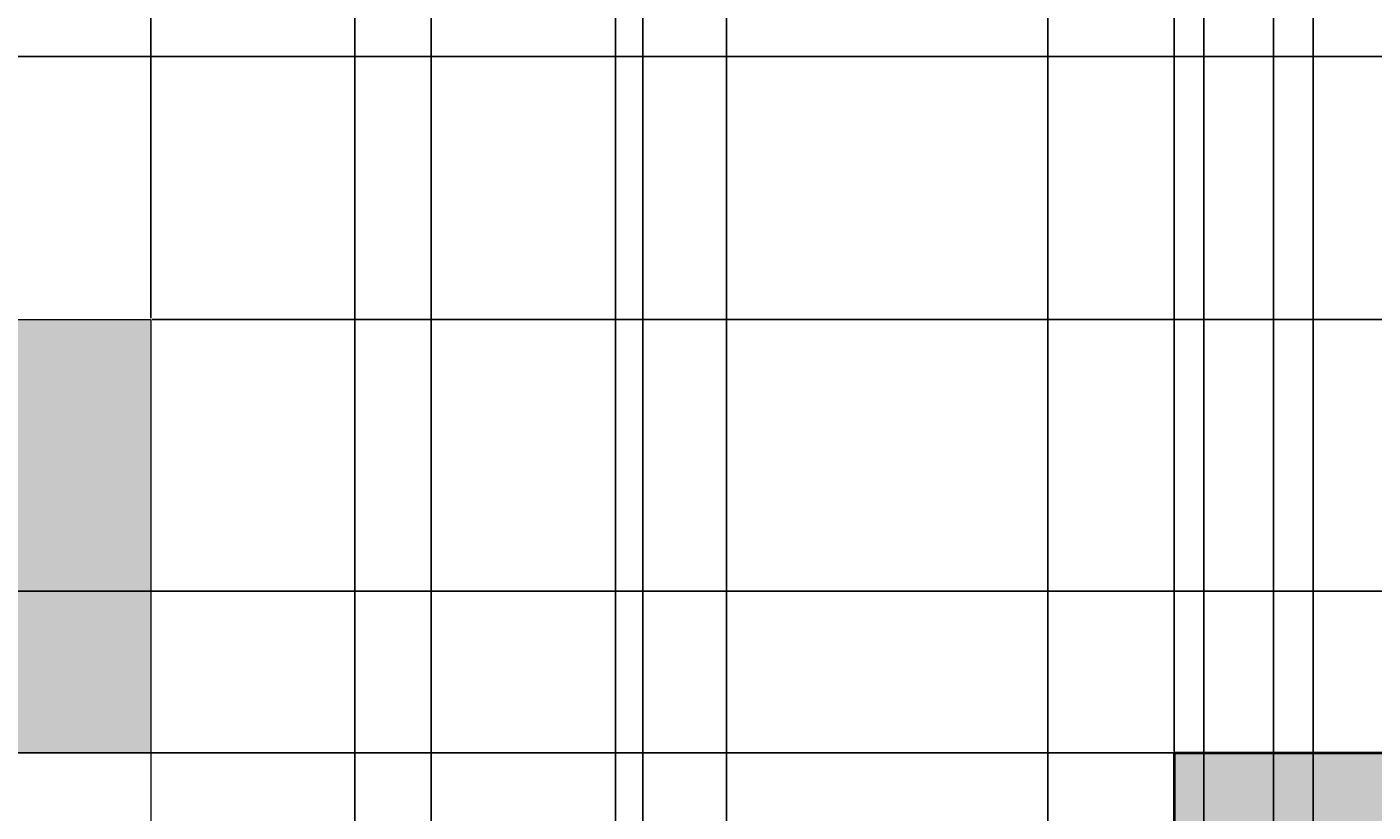
# Model space of a CAD drawing. Units: inches. Extents: x 818 to 1898, y 976 to 2364.
# Tile 70 of 96: x 1372 to 1439, y 1873 to 1913. Entities that reach past the tile are written whole.
import ezdxf

# ---------------------------------------------------------------- set-up
doc = ezdxf.new("R2010")
doc.units = ezdxf.units.IN
doc.header["$LTSCALE"] = 5
doc.header["$MEASUREMENT"] = 0
for name, color, linetype, lineweight in [('A-ANNO-DIMS', 2, 'Continuous', 18), ('A-FLOR-CASE', 8, 'Continuous', 18), ('A-FURN-PATT', 8, 'Continuous', 9), ('A-WALL', 7, 'Continuous', 40)]:
    doc.layers.add(name, color=color, linetype=linetype, lineweight=lineweight)
doc.layers.add('A-WALL-PATT', color=251, linetype='Continuous', lineweight=13, true_color=0x636466)
doc.styles.get("Standard").update_dxf_attribs({"font": 'arial.ttf'})
doc.dimstyles.get("Standard").update_dxf_attribs({"dimtxt": 0.18, "dimasz": 0.18, "dimexe": 0.18, "dimexo": 0.0625, "dimgap": 0.09, "dimtad": 0, "dimtih": 1, "dimtoh": 1, "dimdec": 4, "dimzin": 0, "dimdsep": 46, "dimtxsty": 'Standard', "dimcen": 0.09, "dimadec": 0, "dimazin": 0, "dimtfac": 1, "dimtdec": 4, "dimtofl": 0, "dimtmove": 0, "dimatfit": 3, "dimfxl": 1, "dimtolj": 1, "dimtzin": 0, "dimarcsym": 0})

# ---------------------------------------------------------------- blocks, each defined once
blk = doc.blocks.new('*D61')
at = {"layer": 'A-ANNO-DIMS', "color": 0, "lineweight": -2, "ltscale": 5, "transparency": 16777216}
for p, q in [((1071.725, 1203.027), (1071.725, 2363.873)), ((1071.905, 2363.693), (1250.936, 2363.693)), ((1430.545, 2363.693), (1251.514, 2363.693)), ((1430.725, 1203.027), (1430.725, 2363.873))]:
    blk.add_line(p, q, dxfattribs=at)
at = {"layer": 'A-ANNO-DIMS', "color": 0, "ltscale": 5, "transparency": 16777216}
for points in [[(1071.905, 2363.723), (1071.905, 2363.663), (1071.725, 2363.693)], [(1430.545, 2363.723), (1430.545, 2363.663), (1430.725, 2363.693)]]:
    blk.add_solid(points, dxfattribs=at)
at = {"layer": 'Defpoints', "color": 0, "ltscale": 5, "transparency": 16777216}
for p in [(1430.725, 2363.693), (1071.725, 1202.964), (1430.725, 1202.964)]:
    blk.add_point(p, dxfattribs=at)
at = {"layer": 'A-ANNO-DIMS', "color": 0, "ltscale": 5, "transparency": 16777216, "insert": (1251.225, 2363.693), "char_height": 0.18, "attachment_point": 5}
blk.add_mtext('\\A1;359', dxfattribs=at)
blk = doc.blocks.new('*D64')
at = {"layer": 'A-ANNO-DIMS', "color": 0, "lineweight": -2, "ltscale": 5, "transparency": 16777216}
for p, q in [((1197.725, 1501.141), (1197.725, 2363.873)), ((1197.905, 2363.693), (1313.935, 2363.693)), ((1430.545, 2363.693), (1314.516, 2363.693)), ((1430.725, 1501.141), (1430.725, 2363.873))]:
    blk.add_line(p, q, dxfattribs=at)
at = {"layer": 'A-ANNO-DIMS', "color": 0, "ltscale": 5, "transparency": 16777216}
for points in [[(1197.905, 2363.723), (1197.905, 2363.663), (1197.725, 2363.693)], [(1430.545, 2363.723), (1430.545, 2363.663), (1430.725, 2363.693)]]:
    blk.add_solid(points, dxfattribs=at)
at = {"layer": 'Defpoints', "color": 0, "ltscale": 5, "transparency": 16777216}
for p in [(1430.725, 2363.693), (1197.725, 1501.078), (1430.725, 1501.078)]:
    blk.add_point(p, dxfattribs=at)
at = {"layer": 'A-ANNO-DIMS', "color": 0, "ltscale": 5, "transparency": 16777216, "insert": (1314.225, 2363.693), "char_height": 0.18, "attachment_point": 5}
blk.add_mtext('\\A1;233', dxfattribs=at)
blk = doc.blocks.new('*D74')
at = {"layer": 'A-ANNO-DIMS', "color": 0, "lineweight": -2, "ltscale": 5, "transparency": 16777216}
for p, q in [((1590.663, 1940.078), (818.026, 1940.078)), ((818.206, 1939.898), (818.206, 1925.76)), ((818.206, 1911.258), (818.206, 1925.396)), ((1590.663, 1911.078), (818.026, 1911.078))]:
    blk.add_line(p, q, dxfattribs=at)
at = {"layer": 'A-ANNO-DIMS', "color": 0, "ltscale": 5, "transparency": 16777216}
for points in [[(818.176, 1939.898), (818.236, 1939.898), (818.206, 1940.078)], [(818.176, 1911.258), (818.236, 1911.258), (818.206, 1911.078)]]:
    blk.add_solid(points, dxfattribs=at)
at = {"layer": 'Defpoints', "color": 0, "ltscale": 5, "transparency": 16777216}
for p in [(818.206, 1940.078), (1590.725, 1940.078), (1590.725, 1911.078)]:
    blk.add_point(p, dxfattribs=at)
at = {"layer": 'A-ANNO-DIMS', "color": 0, "ltscale": 5, "transparency": 16777216, "insert": (818.206, 1925.578), "char_height": 0.18, "attachment_point": 5}
blk.add_mtext('\\A1;29', dxfattribs=at)
blk = doc.blocks.new('*D85')
at = {"layer": 'A-ANNO-DIMS', "color": 0, "lineweight": -2, "ltscale": 5, "transparency": 16777216}
for p, q in [((1258.788, 2053.078), (1897.916, 2053.078)), ((1897.736, 2052.898), (1897.736, 1876.76)), ((1897.736, 1700.258), (1897.736, 1876.396)), ((1258.788, 1700.078), (1897.916, 1700.078))]:
    blk.add_line(p, q, dxfattribs=at)
at = {"layer": 'A-ANNO-DIMS', "color": 0, "ltscale": 5, "transparency": 16777216}
for points in [[(1897.706, 2052.898), (1897.766, 2052.898), (1897.736, 2053.078)], [(1897.706, 1700.258), (1897.766, 1700.258), (1897.736, 1700.078)]]:
    blk.add_solid(points, dxfattribs=at)
at = {"layer": 'Defpoints', "color": 0, "ltscale": 5, "transparency": 16777216}
for p in [(1258.725, 2053.078), (1897.736, 2053.078), (1258.725, 1700.078)]:
    blk.add_point(p, dxfattribs=at)
at = {"layer": 'A-ANNO-DIMS', "color": 0, "ltscale": 5, "transparency": 16777216, "insert": (1897.736, 1876.578), "char_height": 0.18, "attachment_point": 5}
blk.add_mtext('\\A1;353', dxfattribs=at)
blk = doc.blocks.new('*D98')
at = {"layer": 'A-ANNO-DIMS', "color": 0, "lineweight": -2, "ltscale": 5, "transparency": 16777216}
for p, q in [((1338.541, 1071.118), (1338.541, 2363.873)), ((1338.721, 2363.693), (1364.815, 2363.693)), ((1391.696, 2363.693), (1365.602, 2363.693)), ((1391.876, 1071.118), (1391.876, 2363.873))]:
    blk.add_line(p, q, dxfattribs=at)
at = {"layer": 'A-ANNO-DIMS', "color": 0, "ltscale": 5, "transparency": 16777216}
for points in [[(1338.721, 2363.723), (1338.721, 2363.663), (1338.541, 2363.693)], [(1391.696, 2363.723), (1391.696, 2363.663), (1391.876, 2363.693)]]:
    blk.add_solid(points, dxfattribs=at)
at = {"layer": 'Defpoints', "color": 0, "ltscale": 5, "transparency": 16777216}
for p in [(1391.876, 2363.693), (1338.541, 1071.055), (1391.876, 1071.055)]:
    blk.add_point(p, dxfattribs=at)
at = {"layer": 'A-ANNO-DIMS', "color": 0, "ltscale": 5, "transparency": 16777216, "insert": (1365.208, 2363.693), "char_height": 0.18, "attachment_point": 5}
blk.add_mtext('\\A1;53.33', dxfattribs=at)
blk = doc.blocks.new('*D99')
at = {"layer": 'A-ANNO-DIMS', "color": 0, "lineweight": -2, "ltscale": 5, "transparency": 16777216}
for p, q in [((1391.876, 1071.118), (1391.876, 2363.873)), ((1392.056, 2363.693), (1420.454, 2363.693)), ((1449.64, 2363.693), (1421.241, 2363.693)), ((1449.82, 1071.118), (1449.82, 2363.873))]:
    blk.add_line(p, q, dxfattribs=at)
at = {"layer": 'A-ANNO-DIMS', "color": 0, "ltscale": 5, "transparency": 16777216}
for points in [[(1392.056, 2363.723), (1392.056, 2363.663), (1391.876, 2363.693)], [(1449.64, 2363.723), (1449.64, 2363.663), (1449.82, 2363.693)]]:
    blk.add_solid(points, dxfattribs=at)
at = {"layer": 'Defpoints', "color": 0, "ltscale": 5, "transparency": 16777216}
for p in [(1449.82, 2363.693), (1391.876, 1071.055), (1449.82, 1071.055)]:
    blk.add_point(p, dxfattribs=at)
at = {"layer": 'A-ANNO-DIMS', "color": 0, "ltscale": 5, "transparency": 16777216, "insert": (1420.848, 2363.693), "char_height": 0.18, "attachment_point": 5}
blk.add_mtext('\\A1;57.94', dxfattribs=at)
blk = doc.blocks.new('*D121')
at = {"layer": 'A-ANNO-DIMS', "color": 0, "lineweight": -2, "ltscale": 5, "transparency": 16777216}
for p, q in [((1766.29, 1884.203), (818.026, 1884.203)), ((818.206, 1884.023), (818.206, 1841.142)), ((818.206, 1797.897), (818.206, 1840.778)), ((1766.29, 1797.717), (818.026, 1797.717))]:
    blk.add_line(p, q, dxfattribs=at)
at = {"layer": 'A-ANNO-DIMS', "color": 0, "ltscale": 5, "transparency": 16777216}
for points in [[(818.176, 1884.023), (818.236, 1884.023), (818.206, 1884.203)], [(818.176, 1797.897), (818.236, 1797.897), (818.206, 1797.717)]]:
    blk.add_solid(points, dxfattribs=at)
at = {"layer": 'Defpoints', "color": 0, "ltscale": 5, "transparency": 16777216}
for p in [(818.206, 1884.203), (1766.352, 1884.203), (1766.352, 1797.717)]:
    blk.add_point(p, dxfattribs=at)
at = {"layer": 'A-ANNO-DIMS', "color": 0, "ltscale": 5, "transparency": 16777216, "insert": (818.206, 1840.96), "char_height": 0.18, "attachment_point": 5}
blk.add_mtext('\\A1;86.49', dxfattribs=at)
blk = doc.blocks.new('*D161')
at = {"layer": 'A-ANNO-DIMS', "color": 0, "lineweight": -2, "ltscale": 5, "transparency": 16777216}
for p, q in [((1429.225, 1876.141), (1429.225, 2363.873)), ((1429.405, 2363.693), (1509.589, 2363.693)), ((1590.545, 2363.693), (1510.361, 2363.693)), ((1590.725, 1876.141), (1590.725, 2363.873))]:
    blk.add_line(p, q, dxfattribs=at)
at = {"layer": 'A-ANNO-DIMS', "color": 0, "ltscale": 5, "transparency": 16777216}
for points in [[(1429.405, 2363.723), (1429.405, 2363.663), (1429.225, 2363.693)], [(1590.545, 2363.723), (1590.545, 2363.663), (1590.725, 2363.693)]]:
    blk.add_solid(points, dxfattribs=at)
at = {"layer": 'Defpoints', "color": 0, "ltscale": 5, "transparency": 16777216}
for p in [(1590.725, 2363.693), (1429.225, 1876.078), (1590.725, 1876.078)]:
    blk.add_point(p, dxfattribs=at)
at = {"layer": 'A-ANNO-DIMS', "color": 0, "ltscale": 5, "transparency": 16777216, "insert": (1509.975, 2363.693), "char_height": 0.18, "attachment_point": 5}
blk.add_mtext('\\A1;161.5', dxfattribs=at)
blk = doc.blocks.new('*D162')
at = {"layer": 'A-ANNO-DIMS', "color": 0, "lineweight": -2, "ltscale": 5, "transparency": 16777216}
for p, q in [((1429.163, 1876.078), (818.026, 1876.078)), ((818.206, 1875.898), (818.206, 1871.76)), ((818.206, 1867.258), (818.206, 1871.396)), ((1429.163, 1867.078), (818.026, 1867.078))]:
    blk.add_line(p, q, dxfattribs=at)
at = {"layer": 'A-ANNO-DIMS', "color": 0, "ltscale": 5, "transparency": 16777216}
for points in [[(818.176, 1875.898), (818.236, 1875.898), (818.206, 1876.078)], [(818.176, 1867.258), (818.236, 1867.258), (818.206, 1867.078)]]:
    blk.add_solid(points, dxfattribs=at)
at = {"layer": 'Defpoints', "color": 0, "ltscale": 5, "transparency": 16777216}
for p in [(1429.225, 1876.078), (818.206, 1867.078), (1429.225, 1867.078)]:
    blk.add_point(p, dxfattribs=at)
at = {"layer": 'A-ANNO-DIMS', "color": 0, "ltscale": 5, "transparency": 16777216, "insert": (818.206, 1871.578), "char_height": 0.18, "attachment_point": 5}
blk.add_mtext('\\A1;9', dxfattribs=at)
blk = doc.blocks.new('*D166')
at = {"layer": 'A-ANNO-DIMS', "color": 0, "lineweight": -2, "ltscale": 5, "transparency": 16777216}
for p, q in [((1401.146, 1510.141), (1401.146, 2363.873)), ((1401.326, 2363.693), (1415.54, 2363.693)), ((1430.545, 2363.693), (1416.331, 2363.693)), ((1430.725, 1510.141), (1430.725, 2363.873))]:
    blk.add_line(p, q, dxfattribs=at)
at = {"layer": 'A-ANNO-DIMS', "color": 0, "ltscale": 5, "transparency": 16777216}
for points in [[(1401.326, 2363.723), (1401.326, 2363.663), (1401.146, 2363.693)], [(1430.545, 2363.723), (1430.545, 2363.663), (1430.725, 2363.693)]]:
    blk.add_solid(points, dxfattribs=at)
at = {"layer": 'Defpoints', "color": 0, "ltscale": 5, "transparency": 16777216}
for p in [(1430.725, 2363.693), (1401.146, 1510.078), (1430.725, 1510.078)]:
    blk.add_point(p, dxfattribs=at)
at = {"layer": 'A-ANNO-DIMS', "color": 0, "ltscale": 5, "transparency": 16777216, "insert": (1415.936, 2363.693), "char_height": 0.18, "attachment_point": 5}
blk.add_mtext('\\A1;29.58', dxfattribs=at)
blk = doc.blocks.new('*D191')
at = {"layer": 'A-ANNO-DIMS', "color": 0, "lineweight": -2, "ltscale": 5, "transparency": 16777216}
for p, q in [((1434.225, 1409.115), (1434.225, 2363.873)), ((1434.405, 2363.693), (1435.076, 2363.693)), ((1436.045, 2363.693), (1435.375, 2363.693)), ((1436.225, 1409.115), (1436.225, 2363.873))]:
    blk.add_line(p, q, dxfattribs=at)
at = {"layer": 'A-ANNO-DIMS', "color": 0, "ltscale": 5, "transparency": 16777216}
for points in [[(1434.405, 2363.723), (1434.405, 2363.663), (1434.225, 2363.693)], [(1436.045, 2363.723), (1436.045, 2363.663), (1436.225, 2363.693)]]:
    blk.add_solid(points, dxfattribs=at)
at = {"layer": 'Defpoints', "color": 0, "ltscale": 5, "transparency": 16777216}
for p in [(1436.225, 2363.693), (1434.225, 1409.052), (1436.225, 1409.052)]:
    blk.add_point(p, dxfattribs=at)
at = {"layer": 'A-ANNO-DIMS', "color": 0, "ltscale": 5, "transparency": 16777216, "insert": (1435.225, 2363.693), "char_height": 0.18, "attachment_point": 5}
blk.add_mtext('\\A1;2', dxfattribs=at)
blk = doc.blocks.new('*D206')
at = {"layer": 'A-ANNO-DIMS', "color": 0, "lineweight": -2, "ltscale": 5, "transparency": 16777216}
for p, q in [((1590.663, 1911.078), (818.026, 1911.078)), ((818.206, 1910.898), (818.206, 1893.76)), ((818.206, 1876.258), (818.206, 1893.396)), ((1590.663, 1876.078), (818.026, 1876.078))]:
    blk.add_line(p, q, dxfattribs=at)
at = {"layer": 'A-ANNO-DIMS', "color": 0, "ltscale": 5, "transparency": 16777216}
for points in [[(818.176, 1910.898), (818.236, 1910.898), (818.206, 1911.078)], [(818.176, 1876.258), (818.236, 1876.258), (818.206, 1876.078)]]:
    blk.add_solid(points, dxfattribs=at)
at = {"layer": 'Defpoints', "color": 0, "ltscale": 5, "transparency": 16777216}
for p in [(818.206, 1911.078), (1590.725, 1911.078), (1590.725, 1876.078)]:
    blk.add_point(p, dxfattribs=at)
at = {"layer": 'A-ANNO-DIMS', "color": 0, "ltscale": 5, "transparency": 16777216, "insert": (818.206, 1893.578), "char_height": 0.18, "attachment_point": 5}
blk.add_mtext('\\A1;35', dxfattribs=at)
blk = doc.blocks.new('*D215')
at = {"layer": 'A-ANNO-DIMS', "color": 0, "lineweight": -2, "ltscale": 5, "transparency": 16777216}
for p, q in [((1590.663, 1876.078), (818.026, 1876.078)), ((818.206, 1875.898), (818.206, 1781.76)), ((818.206, 1687.258), (818.206, 1781.396)), ((1511.663, 1687.078), (818.026, 1687.078))]:
    blk.add_line(p, q, dxfattribs=at)
at = {"layer": 'A-ANNO-DIMS', "color": 0, "ltscale": 5, "transparency": 16777216}
for points in [[(818.176, 1875.898), (818.236, 1875.898), (818.206, 1876.078)], [(818.176, 1687.258), (818.236, 1687.258), (818.206, 1687.078)]]:
    blk.add_solid(points, dxfattribs=at)
at = {"layer": 'Defpoints', "color": 0, "ltscale": 5, "transparency": 16777216}
for p in [(818.206, 1876.078), (1590.725, 1876.078), (1511.725, 1687.078)]:
    blk.add_point(p, dxfattribs=at)
at = {"layer": 'A-ANNO-DIMS', "color": 0, "ltscale": 5, "transparency": 16777216, "insert": (818.206, 1781.578), "char_height": 0.18, "attachment_point": 5}
blk.add_mtext('\\A1;189', dxfattribs=at)
blk = doc.blocks.new('*D231')
at = {"layer": 'A-ANNO-DIMS', "color": 0, "lineweight": -2, "ltscale": 5, "transparency": 16777216}
for p, q in [((1303.931, 1952.978), (1303.931, 975.663)), ((1402.518, 1952.978), (1402.518, 975.663)), ((1304.111, 975.843), (1352.831, 975.843)), ((1402.338, 975.843), (1353.619, 975.843))]:
    blk.add_line(p, q, dxfattribs=at)
at = {"layer": 'A-ANNO-DIMS', "color": 0, "ltscale": 5, "transparency": 16777216}
for points in [[(1304.111, 975.873), (1304.111, 975.813), (1303.931, 975.843)], [(1402.338, 975.873), (1402.338, 975.813), (1402.518, 975.843)]]:
    blk.add_solid(points, dxfattribs=at)
at = {"layer": 'Defpoints', "color": 0, "ltscale": 5, "transparency": 16777216}
for p in [(1303.931, 1953.041), (1402.518, 1953.041), (1402.518, 975.843)]:
    blk.add_point(p, dxfattribs=at)
at = {"layer": 'A-ANNO-DIMS', "color": 0, "ltscale": 5, "transparency": 16777216, "insert": (1353.225, 975.843), "char_height": 0.18, "attachment_point": 5}
blk.add_mtext('\\A1;98.59', dxfattribs=at)
blk = doc.blocks.new('*D252')
at = {"layer": 'A-ANNO-DIMS', "color": 0, "lineweight": -2, "ltscale": 5, "transparency": 16777216}
for p, q in [((1330.305, 2053.016), (1330.305, 975.663)), ((1388.031, 2053.016), (1388.031, 975.663)), ((1330.485, 975.843), (1358.775, 975.843)), ((1387.851, 975.843), (1359.562, 975.843))]:
    blk.add_line(p, q, dxfattribs=at)
at = {"layer": 'A-ANNO-DIMS', "color": 0, "ltscale": 5, "transparency": 16777216}
for points in [[(1330.485, 975.873), (1330.485, 975.813), (1330.305, 975.843)], [(1387.851, 975.873), (1387.851, 975.813), (1388.031, 975.843)]]:
    blk.add_solid(points, dxfattribs=at)
at = {"layer": 'Defpoints', "color": 0, "ltscale": 5, "transparency": 16777216}
for p in [(1330.305, 2053.078), (1388.031, 2053.078), (1388.031, 975.843)]:
    blk.add_point(p, dxfattribs=at)
at = {"layer": 'A-ANNO-DIMS', "color": 0, "ltscale": 5, "transparency": 16777216, "insert": (1359.168, 975.843), "char_height": 0.18, "attachment_point": 5}
blk.add_mtext('\\A1;57.73', dxfattribs=at)
blk = doc.blocks.new('*D273')
at = {"layer": 'A-ANNO-DIMS', "color": 0, "lineweight": -2, "ltscale": 5, "transparency": 16777216}
for p, q in [((1406.725, 1587.479), (1406.725, 2363.873)), ((1406.905, 2363.693), (1418.505, 2363.693)), ((1430.545, 2363.693), (1418.945, 2363.693)), ((1430.725, 1587.479), (1430.725, 2363.873))]:
    blk.add_line(p, q, dxfattribs=at)
at = {"layer": 'A-ANNO-DIMS', "color": 0, "ltscale": 5, "transparency": 16777216}
for points in [[(1406.905, 2363.723), (1406.905, 2363.663), (1406.725, 2363.693)], [(1430.545, 2363.723), (1430.545, 2363.663), (1430.725, 2363.693)]]:
    blk.add_solid(points, dxfattribs=at)
at = {"layer": 'Defpoints', "color": 0, "ltscale": 5, "transparency": 16777216}
for p in [(1430.725, 2363.693), (1406.725, 1587.416), (1430.725, 1587.416)]:
    blk.add_point(p, dxfattribs=at)
at = {"layer": 'A-ANNO-DIMS', "color": 0, "ltscale": 5, "transparency": 16777216, "insert": (1418.725, 2363.693), "char_height": 0.18, "attachment_point": 5}
blk.add_mtext('\\A1;24', dxfattribs=at)
blk = doc.blocks.new('*D274')
at = {"layer": 'A-ANNO-DIMS', "color": 0, "lineweight": -2, "ltscale": 5, "transparency": 16777216}
for p, q in [((1311.025, 1897.929), (1311.025, 2363.873)), ((1311.205, 2363.693), (1344.007, 2363.693)), ((1377.599, 2363.693), (1344.797, 2363.693)), ((1377.779, 1897.929), (1377.779, 2363.873))]:
    blk.add_line(p, q, dxfattribs=at)
at = {"layer": 'A-ANNO-DIMS', "color": 0, "ltscale": 5, "transparency": 16777216}
for points in [[(1311.205, 2363.723), (1311.205, 2363.663), (1311.025, 2363.693)], [(1377.599, 2363.723), (1377.599, 2363.663), (1377.779, 2363.693)]]:
    blk.add_solid(points, dxfattribs=at)
at = {"layer": 'Defpoints', "color": 0, "ltscale": 5, "transparency": 16777216}
for p in [(1377.779, 2363.693), (1311.025, 1897.866), (1377.779, 1897.866)]:
    blk.add_point(p, dxfattribs=at)
at = {"layer": 'A-ANNO-DIMS', "color": 0, "ltscale": 5, "transparency": 16777216, "insert": (1344.402, 2363.693), "char_height": 0.18, "attachment_point": 5}
blk.add_mtext('\\A1;66.75', dxfattribs=at)
blk = doc.blocks.new('*D275')
at = {"layer": 'A-ANNO-DIMS', "color": 0, "lineweight": -2, "ltscale": 5, "transparency": 16777216}
for p, q in [((1377.842, 1897.866), (1897.916, 1897.866)), ((1897.736, 1897.686), (1897.736, 1875.988)), ((1897.736, 1853.93), (1897.736, 1875.628)), ((1377.842, 1853.75), (1897.916, 1853.75))]:
    blk.add_line(p, q, dxfattribs=at)
at = {"layer": 'A-ANNO-DIMS', "color": 0, "ltscale": 5, "transparency": 16777216}
for points in [[(1897.706, 1897.686), (1897.766, 1897.686), (1897.736, 1897.866)], [(1897.706, 1853.93), (1897.766, 1853.93), (1897.736, 1853.75)]]:
    blk.add_solid(points, dxfattribs=at)
at = {"layer": 'Defpoints', "color": 0, "ltscale": 5, "transparency": 16777216}
for p in [(1377.779, 1897.866), (1897.736, 1897.866), (1377.779, 1853.75)]:
    blk.add_point(p, dxfattribs=at)
at = {"layer": 'A-ANNO-DIMS', "color": 0, "ltscale": 5, "transparency": 16777216, "insert": (1897.736, 1875.808), "char_height": 0.18, "attachment_point": 5}
blk.add_mtext('\\A1;44.12', dxfattribs=at)
blk = doc.blocks.new('*D282')
at = {"layer": 'A-ANNO-DIMS', "color": 0, "lineweight": -2, "ltscale": 5, "transparency": 16777216}
for p, q in [((1422.083, 2081.188), (1897.916, 2081.188)), ((1897.736, 2081.008), (1897.736, 1884.315)), ((1897.736, 1687.258), (1897.736, 1883.951)), ((1463.788, 1687.078), (1897.916, 1687.078))]:
    blk.add_line(p, q, dxfattribs=at)
at = {"layer": 'A-ANNO-DIMS', "color": 0, "ltscale": 5, "transparency": 16777216}
for points in [[(1897.706, 2081.008), (1897.766, 2081.008), (1897.736, 2081.188)], [(1897.706, 1687.258), (1897.766, 1687.258), (1897.736, 1687.078)]]:
    blk.add_solid(points, dxfattribs=at)
at = {"layer": 'Defpoints', "color": 0, "ltscale": 5, "transparency": 16777216}
for p in [(1422.02, 2081.188), (1897.736, 2081.188), (1463.725, 1687.078)]:
    blk.add_point(p, dxfattribs=at)
at = {"layer": 'A-ANNO-DIMS', "color": 0, "ltscale": 5, "transparency": 16777216, "insert": (1897.736, 1884.133), "char_height": 0.18, "attachment_point": 5}
blk.add_mtext('\\A1;394.1', dxfattribs=at)
blk = doc.blocks.new('*D288')
at = {"layer": 'A-ANNO-DIMS', "color": 0, "lineweight": -2, "ltscale": 5, "transparency": 16777216}
for p, q in [((1422.876, 1742.674), (1422.876, 2363.873)), ((1423.056, 2363.693), (1466.906, 2363.693)), ((1511.545, 2363.693), (1467.695, 2363.693)), ((1511.725, 1716.108), (1511.725, 2363.873))]:
    blk.add_line(p, q, dxfattribs=at)
at = {"layer": 'A-ANNO-DIMS', "color": 0, "ltscale": 5, "transparency": 16777216}
for points in [[(1423.056, 2363.723), (1423.056, 2363.663), (1422.876, 2363.693)], [(1511.545, 2363.723), (1511.545, 2363.663), (1511.725, 2363.693)]]:
    blk.add_solid(points, dxfattribs=at)
at = {"layer": 'Defpoints', "color": 0, "ltscale": 5, "transparency": 16777216}
for p in [(1511.725, 2363.693), (1422.876, 1742.611), (1511.725, 1716.045)]:
    blk.add_point(p, dxfattribs=at)
at = {"layer": 'A-ANNO-DIMS', "color": 0, "ltscale": 5, "transparency": 16777216, "insert": (1467.3, 2363.693), "char_height": 0.18, "attachment_point": 5}
blk.add_mtext('\\A1;88.85', dxfattribs=at)

msp = doc.modelspace()

# ---------------------------------------------------------------- hatches: boundary and pattern name
at = {"layer": 'A-FURN-PATT', "ltscale": 5}
h = msp.add_hatch(color=256, dxfattribs=at)
h.dxf.hatch_style = 1
h.paths.add_polyline_path([(1336.7936, 1953.0408), (1314.2595, 1953.0408), (1314.2595, 1941.0096), (1336.7936, 1941.0096)])
h.paths.add_polyline_path([(1338.9915, 1941.0096), (1336.7936, 1941.0096), (1336.7936, 1937.7177), (1314.2595, 1937.7177), (1314.2595, 1941.0096), (1310.9077, 1941.0096), (1310.9077, 1935.2252), (1338.9915, 1935.2252)])
h.paths.add_polyline_path([(1336.7936, 1941.0096), (1314.2595, 1941.0096), (1314.2595, 1937.7177), (1336.7936, 1937.7177)], flags=17)
h.paths.add_polyline_path([(1367.9307, 1959.6079), (1345.3966, 1959.6079), (1345.3966, 1941.0096), (1367.9307, 1941.0096)])
h.paths.add_polyline_path([(1398.8475, 1953.0408), (1376.3134, 1953.0408), (1376.3134, 1952.6393), (1390.1242, 1941.0096), (1398.8475, 1941.0096)])
h.paths.add_polyline_path([(1376.3134, 1952.6393), (1376.3134, 1941.0096), (1390.1242, 1941.0096)], flags=17)
h.paths.add_polyline_path([(1370.1286, 1941.0096), (1367.9307, 1941.0096), (1367.9307, 1937.7177), (1345.3966, 1937.7177), (1345.3966, 1941.0096), (1342.0448, 1941.0096), (1342.0448, 1935.2252), (1370.1286, 1935.2252)])
h.paths.add_polyline_path([(1367.9307, 1941.0096), (1345.3966, 1941.0096), (1345.3966, 1937.7177), (1367.9307, 1937.7177)], flags=17)
h.paths.add_polyline_path([(1390.1242, 1941.0096), (1376.3134, 1941.0096), (1376.3134, 1937.7177), (1394.0336, 1937.7177)], flags=17)
h.paths.add_polyline_path([(1394.0336, 1937.7177), (1376.3134, 1937.7177), (1376.3134, 1941.0096), (1372.9616, 1941.0096), (1372.9616, 1935.2252), (1396.9935, 1935.2252)])
h.paths.add_polyline_path([(1398.8475, 1941.0096), (1390.1242, 1941.0096), (1394.0336, 1937.7177), (1398.8475, 1937.7177)])
h.paths.add_polyline_path([(1401.0455, 1941.0096), (1398.8475, 1941.0096), (1398.8475, 1937.7177), (1394.0336, 1937.7177), (1396.9935, 1935.2252), (1401.0455, 1935.2252)])
h.paths.add_polyline_path([(1336.7936, 2020.4229), (1314.2595, 2020.4229), (1314.2595, 2008.3917), (1336.7936, 2008.3917)])
h.paths.add_polyline_path([(1336.7936, 2023.7149), (1314.2595, 2023.7149), (1314.2595, 2020.4229), (1336.7936, 2020.4229)], flags=17)
h.paths.add_polyline_path([(1338.9915, 2026.2074), (1310.9077, 2026.2074), (1310.9077, 2020.4229), (1314.2595, 2020.4229), (1314.2595, 2023.7149), (1336.7936, 2023.7149), (1336.7936, 2020.4229), (1338.9915, 2020.4229)])
h.paths.add_polyline_path([(1367.9307, 2023.7149), (1345.3966, 2023.7149), (1345.3966, 2020.4229), (1367.9307, 2020.4229)], flags=17)
h.paths.add_polyline_path([(1370.1286, 2026.2074), (1342.0448, 2026.2074), (1342.0448, 2020.4229), (1345.3966, 2020.4229), (1345.3966, 2023.7149), (1367.9307, 2023.7149), (1367.9307, 2020.4229), (1370.1286, 2020.4229)])
h.paths.add_polyline_path([(1367.9307, 2020.4229), (1345.3966, 2020.4229), (1345.3966, 2008.3917), (1367.9307, 2008.3917)])
h.paths.add_polyline_path([(1398.8475, 2020.4229), (1388.1824, 2020.4229), (1376.3134, 2010.4284), (1376.3134, 2008.3917), (1398.8475, 2008.3917)])
h.paths.add_polyline_path([(1392.0918, 2023.7149), (1376.3134, 2023.7149), (1376.3134, 2020.4229), (1388.1824, 2020.4229)], flags=17)
h.paths.add_polyline_path([(1388.1824, 2020.4229), (1376.3134, 2020.4229), (1376.3134, 2010.4284)], flags=17)
h.paths.add_polyline_path([(1395.0518, 2026.2074), (1372.9616, 2026.2074), (1372.9616, 2020.4229), (1376.3134, 2020.4229), (1376.3134, 2023.7149), (1392.0918, 2023.7149)])
h.paths.add_polyline_path([(1398.8475, 2023.7149), (1392.0918, 2023.7149), (1388.1824, 2020.4229), (1398.8475, 2020.4229)])
h.paths.add_polyline_path([(1401.0455, 2026.2074), (1395.0518, 2026.2074), (1392.0918, 2023.7149), (1398.8475, 2023.7149), (1398.8475, 2020.4229), (1401.0455, 2020.4229)])
h.paths.add_polyline_path([(1327.0339, 1897.8663), (1311.025, 1897.8663), (1311.025, 1876.0782), (1327.0339, 1876.0782)])
h.paths.add_polyline_path([(1377.7791, 1897.8663), (1359.9579, 1897.8663), (1359.9579, 1876.0782), (1377.7791, 1876.0782)])
h.paths.add_polyline_path([(1430.7251, 1541.0439), (1406.7251, 1541.0439), (1406.7251, 1525.9965), (1430.7251, 1525.9965)])
h.paths.add_polyline_path([(1430.7251, 1587.4164), (1406.7251, 1587.4164), (1406.7251, 1570.9187), (1430.7251, 1570.9187)])
at = {"layer": 'A-WALL-PATT', "ltscale": 5}
h = msp.add_hatch(color=256, dxfattribs=at)
h.dxf.hatch_style = 1
h.paths.add_polyline_path([(1267.7252, 1928.9218), (1258.7251, 1928.9218), (1258.7251, 1913.6401), (1250.3029, 1913.6401), (1250.3029, 1878.3919), (1258.7251, 1878.3919), (1258.7251, 1862.9652), (1267.7252, 1862.9652)])
h.paths.add_polyline_path([(1267.7252, 1814.9652), (1258.7251, 1814.9652), (1258.7251, 1755.3321), (1267.7252, 1755.3321)])
h.paths.add_polyline_path([(1463.7251, 1696.0782), (1267.7252, 1696.0782), (1267.7252, 1707.3321), (1258.7251, 1707.3321), (1258.7251, 1700.0782), (1251.9333, 1700.0782), (1251.9333, 1687.0782), (1463.7251, 1687.0782)])
h.paths.add_polyline_path([(1714.7252, 1717.3178), (1705.7252, 1717.3178), (1705.7252, 1696.0782), (1599.7252, 1696.0782), (1599.7252, 1790.0782), (1705.7252, 1790.0782), (1705.7252, 1785.6125), (1714.7252, 1785.6125), (1714.7252, 1827.2125), (1705.7252, 1827.2125), (1705.7252, 1802.0782), (1599.7252, 1802.0782), (1599.7252, 1867.0782), (1705.7252, 1867.0782), (1705.7252, 1857.2125), (1714.7252, 1857.2125), (1714.7252, 1930.0316), (1741.8409, 1930.0316), (1741.8409, 1935.0316), (1714.7252, 1935.0316), (1714.7252, 1957.0338), (1741.8409, 1957.0338), (1741.8409, 1962.0338), (1714.7252, 1962.0338), (1705.7252, 1962.0338), (1705.7252, 1948.0782), (1599.7252, 1948.0782), (1599.7252, 1981.0782), (1590.7251, 1981.0782), (1590.7251, 1941.0782), (1620.7252, 1941.0782), (1705.7252, 1941.0782), (1705.7252, 1876.0782), (1599.7252, 1876.0782), (1599.7252, 1911.0782), (1590.7251, 1911.0782), (1590.7251, 1876.0782), (1429.2251, 1876.0782), (1429.2251, 1867.0782), (1511.7251, 1867.0782), (1528.593, 1867.0782), (1595.7252, 1867.0782), (1595.7252, 1773.0782), (1520.7252, 1773.0782), (1520.7252, 1837.5823), (1532.593, 1837.5823), (1532.593, 1867.0782), (1528.593, 1867.0782), (1528.593, 1841.5823), (1511.7251, 1841.5823), (1511.7251, 1744.9714), (1520.7252, 1744.9714), (1520.7252, 1761.0782), (1595.7252, 1761.0782), (1595.7252, 1696.0782), (1520.7252, 1696.0782), (1520.7252, 1716.0454), (1511.7251, 1716.0454), (1511.7251, 1696.0782), (1511.7251, 1687.0782), (1714.7252, 1687.0782)])
h.paths.add_polyline_path([(1714.7252, 2053.0782), (1714.7252, 2081.1881), (1709.7252, 2081.1881), (1709.7252, 2053.0782), (1681.6446, 2053.0782), (1681.6446, 2081.1881), (1676.6446, 2081.1881), (1676.6446, 2053.0782), (1538.5155, 2053.0782), (1538.5155, 2044.0782), (1590.7251, 2044.0782), (1590.7251, 2011.0782), (1599.7252, 2011.0782), (1599.7252, 2044.0782), (1705.7252, 2044.0782), (1705.7252, 2014.5114), (1714.7252, 2014.5114)])
h.paths.add_polyline_path([(1485.1216, 2053.0782), (1422.02, 2053.0782), (1422.02, 2081.1881), (1413.02, 2081.1881), (1413.02, 2053.0782), (1399.6356, 2053.0782), (1399.6356, 2081.1881), (1390.6356, 2081.1881), (1390.6356, 2053.0782), (1388.0315, 2053.0782), (1388.0315, 2044.0782), (1416.2743, 2044.0782), (1485.1216, 2044.0782)])
h.paths.add_polyline_path([(1330.305, 2053.0782), (1258.7251, 2053.0782), (1258.7251, 2019.2871), (1267.7252, 2019.2871), (1267.7252, 2044.0782), (1330.305, 2044.0782)])
h.paths.add_polyline_path([(1258.7251, 2053.0782), (1214.6577, 2053.0782), (1214.6577, 2044.0782), (1258.7251, 2044.0782)])
h.paths.add_polyline_path([(1214.6577, 2053.0782), (1180.349, 2053.0782), (1180.349, 2044.0782), (1214.6577, 2044.0782)])
h.paths.add_polyline_path([(1714.7252, 1639.5782), (1741.8409, 1639.5782), (1741.8409, 1643.5782), (1714.7252, 1643.5782), (1714.7252, 1649.9029), (1705.7252, 1649.9029), (1705.7252, 1600.0782), (1477.7252, 1600.0782), (1477.7252, 1591.0782), (1520.7252, 1591.0782), (1616.7252, 1591.0782), (1616.7252, 1416.6857), (1622.7252, 1416.6857), (1622.7252, 1463.0782), (1624.7252, 1463.0782), (1624.7252, 1467.0782), (1622.7252, 1467.0782), (1622.7252, 1591.0782), (1705.7252, 1591.0782), (1705.7252, 1545.0782), (1714.7252, 1545.0782), (1741.8409, 1545.0782), (1741.8409, 1549.0782), (1714.7252, 1549.0782), (1714.7252, 1593.9175), (1737.8409, 1593.9175), (1737.8409, 1597.9175), (1714.7252, 1597.9175)])
h.paths.add_polyline_path([(1674.9024, 2060.7419), (1714.7045, 2060.7419), (1714.7045, 2073.1061), (1674.9024, 2073.1061)], flags=25)
h.paths.add_polyline_path([(1394.5468, 2061.6618), (1422.2344, 2061.6618), (1422.2344, 2074.0261), (1394.5468, 2074.0261)], flags=24)

# ---------------------------------------------------------------- linework, layer by layer
at = {"layer": 'A-FLOR-CASE'}
for q in [(1311.3271, 1876.0782), (1377.7791, 1867.0782)]:
    msp.add_line((1377.7791, 1876.0782), q, dxfattribs=at)
msp.add_lwpolyline([(1377.7791, 1876.0782), (1311.025, 1876.0782), (1311.025, 1897.8663), (1377.7791, 1897.8663)], close=True, dxfattribs=at)
at = {"layer": 'A-WALL'}
for q in [(1429.2251, 1867.0782), (1590.7251, 1876.0782)]:
    msp.add_line((1429.2251, 1876.0782), q, dxfattribs=at)

# ---------------------------------------------------------------- dimensions: what is measured, and where the dimension line sits
at = {"layer": 'A-ANNO-DIMS', "ltscale": 5}
for base, p1, p2, override, picture, middle in [((1430.7251, 2363.6929), (1071.7251, 1202.9642), (1430.7251, 1202.9642), {"dimdec": 0, "dimlfac": 1, "dimrnd": 0, "dimzin": 0, "dimdsep": 46, "dimlunit": 2}, '*D61', (1251.2251, 2363.6929)), ((1430.7251, 2363.6929), (1197.7251, 1501.0782), (1430.7251, 1501.0782), {"dimdec": 0, "dimlfac": 1, "dimrnd": 0, "dimzin": 0, "dimdsep": 46, "dimlunit": 2}, '*D64', (1314.2251, 2363.6929)), ((1377.7791, 2363.6929), (1311.025, 1897.8663), (1377.7791, 1897.8663), {"dimdec": 2, "dimlfac": 1, "dimrnd": 0, "dimzin": 0, "dimdsep": 46, "dimlunit": 2}, '*D274', (1344.4021, 2363.6929)), ((1391.8757, 2363.6929), (1338.5412, 1071.0552), (1391.8757, 1071.0552), {"dimdec": 2, "dimlfac": 1, "dimrnd": 0, "dimzin": 0, "dimdsep": 46, "dimlunit": 2}, '*D98', (1365.2084, 2363.6929)), ((1449.8196, 2363.6929), (1391.8757, 1071.0552), (1449.8196, 1071.0552), {"dimdec": 2, "dimlfac": 1, "dimrnd": 0, "dimzin": 0, "dimdsep": 46, "dimlunit": 2}, '*D99', (1420.8477, 2363.6929)), ((1430.7251, 2363.6929), (1401.1463, 1510.0782), (1430.7251, 1510.0782), {"dimdec": 2, "dimlfac": 1, "dimrnd": 0, "dimzin": 0, "dimdsep": 46, "dimlunit": 2}, '*D166', (1415.9357, 2363.6929)), ((1430.7251, 2363.6929), (1406.7251, 1587.4164), (1430.7251, 1587.4164), {"dimdec": 0, "dimlfac": 1, "dimrnd": 0, "dimzin": 0, "dimdsep": 46, "dimlunit": 2}, '*D273', (1418.7251, 2363.6929)), ((1511.7251, 2363.6929), (1422.8756, 1742.6113), (1511.7251, 1716.0454), {"dimdec": 2, "dimlfac": 1, "dimrnd": 0, "dimzin": 0, "dimdsep": 46, "dimlunit": 2}, '*D288', (1467.3004, 2363.6929)), ((1590.7251, 2363.6929), (1429.2251, 1876.0782), (1590.7251, 1876.0782), {"dimdec": 1, "dimlfac": 1, "dimrnd": 0, "dimzin": 0, "dimdsep": 46, "dimlunit": 2}, '*D161', (1509.9751, 2363.6929)), ((1436.2251, 2363.6929), (1434.2251, 1409.0522), (1436.2251, 1409.0522), {"dimdec": 0, "dimlfac": 1, "dimrnd": 0, "dimzin": 0, "dimdsep": 46, "dimlunit": 2}, '*D191', (1435.2251, 2363.6929)), ((1388.0315, 975.8433), (1330.305, 2053.0782), (1388.0315, 2053.0782), {"dimdec": 2, "dimlfac": 1, "dimrnd": 0, "dimzin": 0, "dimdsep": 46, "dimlunit": 2}, '*D252', (1359.1682, 975.8433)), ((1402.518, 975.8433), (1303.9314, 1953.0408), (1402.518, 1953.0408), {"dimdec": 2, "dimlfac": 1, "dimrnd": 0, "dimzin": 0, "dimdsep": 46, "dimlunit": 2}, '*D231', (1353.2247, 975.8433))]:
    dim = msp.add_linear_dim(base=base, p1=p1, p2=p2, dimstyle='Standard', override=override, dxfattribs=at)
    dim.commit()
    dim.dimension.update_dxf_attribs({"geometry": picture, "text_midpoint": middle})
for base, p1, p2, override, picture, middle in [((1897.736, 2081.1881), (1463.7251, 1687.0782), (1422.02, 2081.1881), {"dimdec": 1, "dimlfac": 1, "dimrnd": 0, "dimzin": 0, "dimdsep": 46, "dimlunit": 2}, '*D282', (1897.736, 1884.1332)), ((1897.736, 2053.0782), (1258.7251, 1700.0782), (1258.7251, 2053.0782), {"dimdec": 0, "dimlfac": 1, "dimrnd": 0, "dimzin": 0, "dimdsep": 46, "dimlunit": 2}, '*D85', (1897.736, 1876.5782)), ((818.2059, 1940.0782), (1590.7251, 1911.0782), (1590.7251, 1940.0782), {"dimdec": 0, "dimlfac": 1, "dimrnd": 0, "dimzin": 0, "dimdsep": 46, "dimlunit": 2}, '*D74', (818.2059, 1925.5782)), ((818.2059, 1911.0782), (1590.7251, 1876.0782), (1590.7251, 1911.0782), {"dimdec": 0, "dimlfac": 1, "dimrnd": 0, "dimzin": 0, "dimdsep": 46, "dimlunit": 2}, '*D206', (818.2059, 1893.5782)), ((1897.736, 1897.8663), (1377.7791, 1853.7496), (1377.7791, 1897.8663), {"dimdec": 2, "dimlfac": 1, "dimrnd": 0, "dimzin": 0, "dimdsep": 46, "dimlunit": 2}, '*D275', (1897.736, 1875.808)), ((818.2059, 1884.2031), (1766.3524, 1797.7165), (1766.3524, 1884.2031), {"dimdec": 2, "dimlfac": 1, "dimrnd": 0, "dimzin": 0, "dimdsep": 46, "dimlunit": 2}, '*D121', (818.2059, 1840.9598)), ((818.2059, 1876.0782), (1511.7251, 1687.0782), (1590.7251, 1876.0782), {"dimdec": 0, "dimlfac": 1, "dimrnd": 0, "dimzin": 0, "dimdsep": 46, "dimlunit": 2}, '*D215', (818.2059, 1781.5782)), ((818.2059, 1867.0782), (1429.2251, 1876.0782), (1429.2251, 1867.0782), {"dimdec": 0, "dimlfac": 1, "dimrnd": 0, "dimzin": 0, "dimdsep": 46, "dimlunit": 2}, '*D162', (818.2059, 1871.5782))]:
    dim = msp.add_linear_dim(base=base, p1=p1, p2=p2, angle=90, dimstyle='Standard', override=override, dxfattribs=at)
    dim.commit()
    dim.dimension.update_dxf_attribs({"geometry": picture, "text_midpoint": middle})

doc.saveas('drawing.dxf')
